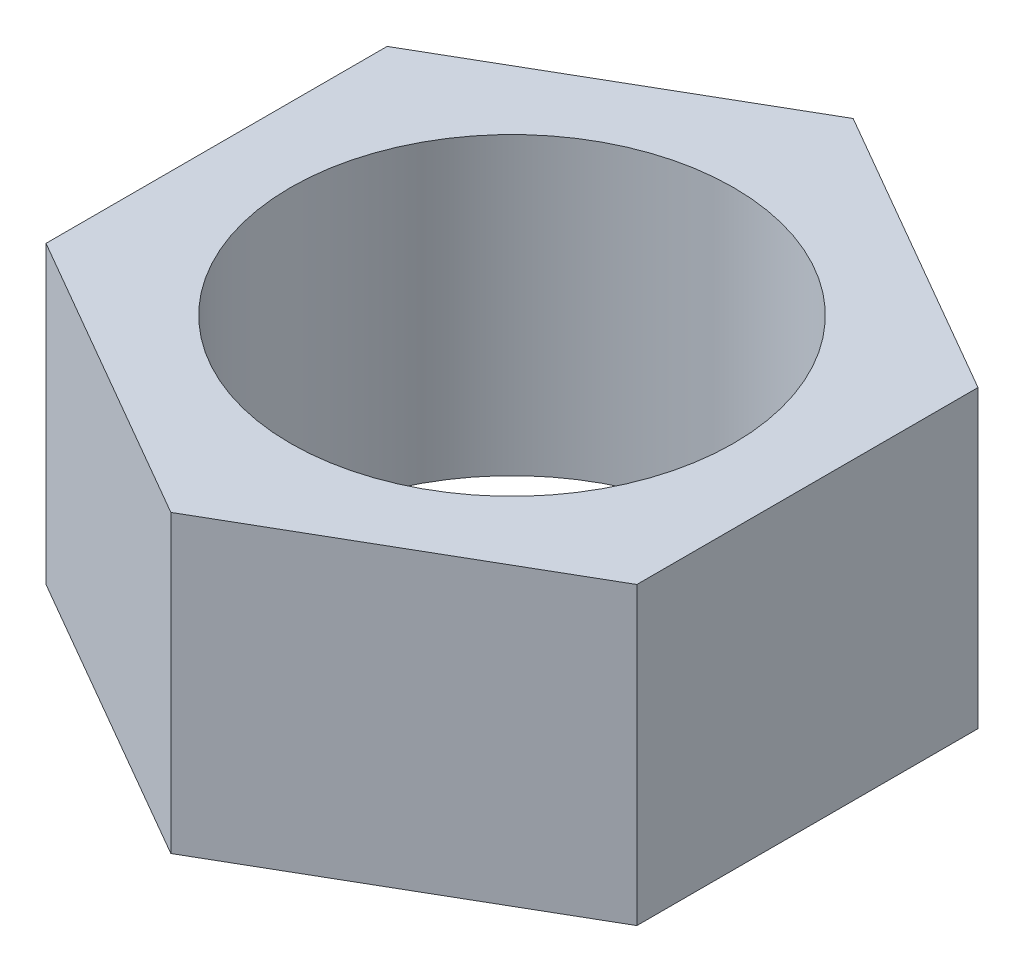
SolidWorks part; units mm, degrees
material "Plain Carbon Steel"
ref_plane "Front Plane" through (0, 0, 0) normal (0, 0, 1) x (1, 0, 0)
ref_plane "Top Plane" through (0, 0, 0) normal (0, 1, 0) x (1, 0, 0)
ref_plane "Right Plane" through (0, 0, 0) normal (1, 0, 0) x (0, 0, -1)
sketch "Hex Profile 16AF with Bore Ø12" plane through (0, 0, 0) normal (0, 1, 0) x (1, 0, 0)
  line L1 (0, -9.2376) -> (8, -4.6188)
  line L2 (8, -4.6188) -> (8, 4.6188)
  line L3 (8, 4.6188) -> (0, 9.2376)
  line L4 (0, 9.2376) -> (-8, 4.6188)
  line L5 (-8, 4.6188) -> (-8, -4.6188)
  line L6 (-8, -4.6188) -> (0, -9.2376)
  circle A0 centre (0, 0) radius 8 construction
  circle A1 centre (0, 0) radius 6
  dimension "D2" = 12
  dimension "D1" = 16
extrude "Nut Body 8 mm" add sketch "Hex Profile 16AF with Bore Ø12" along normal mid plane 8
